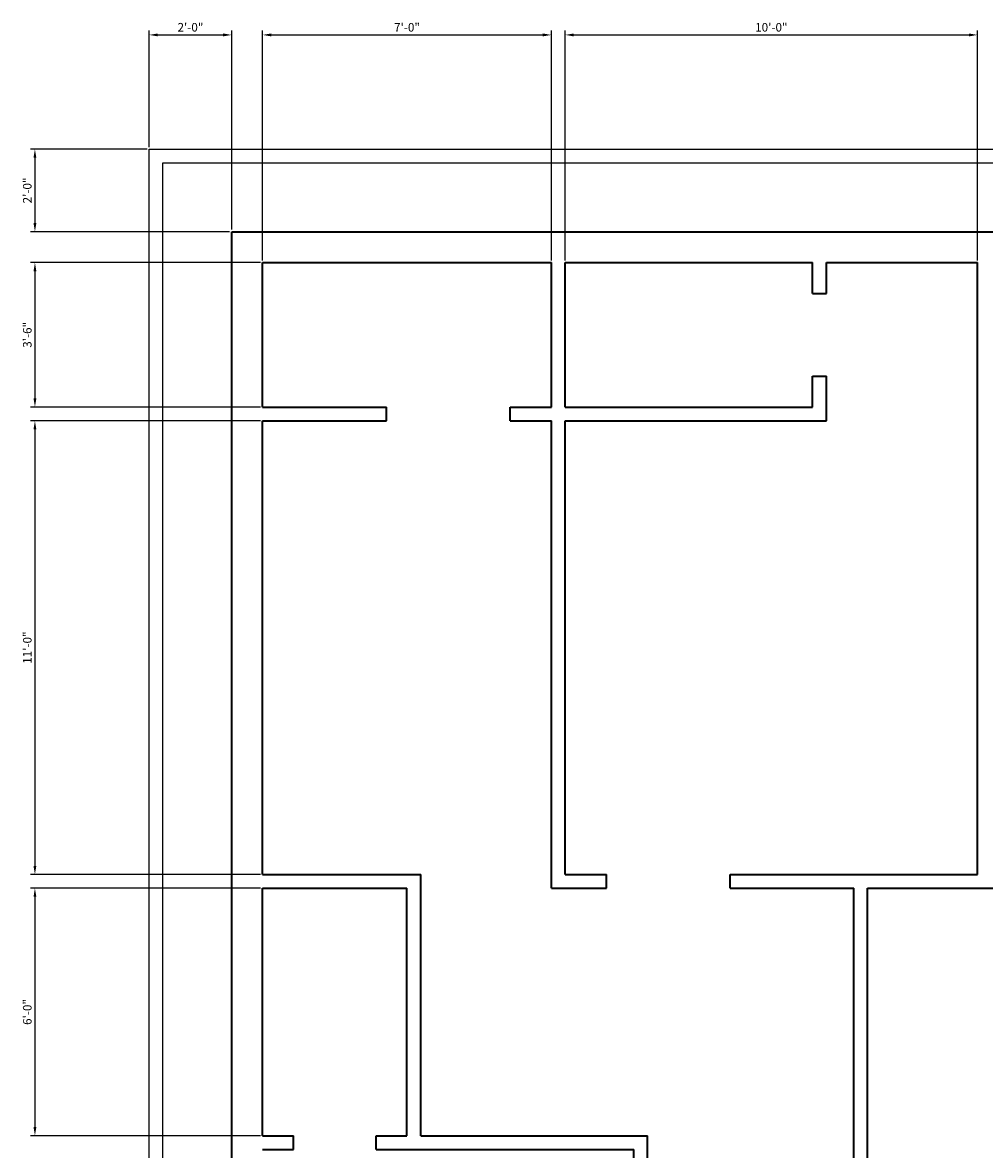
# Model space of a CAD drawing. Units: inches. Extents: x 2169 to 10664, y 1669 to 6352.
# Tile 11 of 17: x 4397 to 4677, y 2329 to 2657. Entities that reach past the tile are written whole.
import ezdxf

# ---------------------------------------------------------------- set-up
doc = ezdxf.new("R2010")
doc.units = ezdxf.units.IN
for name, color, linetype, lineweight in [('A-ANNO-DIMS', 3, 'Continuous', 18), ('A-WALL', 7, 'Continuous', 35), ('C-PROP', 251, 'Continuous', 25)]:
    doc.layers.add(name, color=color, linetype=linetype, lineweight=lineweight)
doc.styles.get("Standard").update_dxf_attribs({"font": 'arial.ttf'})
doc.dimstyles.new('ISO-25', dxfattribs={"dimtxt": 2.5, "dimasz": 2.5, "dimexe": 1.25, "dimexo": 0.625, "dimtad": 1, "dimdec": 0, "dimlunit": 3, "dimtxsty": 'Standard', "dimcen": 2.5, "dimadec": 0, "dimazin": 0, "dimtfac": 1, "dimtdec": 0, "dimtmove": 0, "dimatfit": 3, "dimfxl": 1, "dimarcsym": 0})

# ---------------------------------------------------------------- blocks, each defined once
blk = doc.blocks.new('*D104')
at = {"layer": 'A-ANNO-DIMS', "color": 0, "lineweight": -2, "transparency": 16777216}
for p, q in [((4433.57, 2620.81), (4433.57, 2654.69)), ((4436.07, 2653.44), (4455.07, 2653.44)), ((4457.57, 2596.81), (4457.57, 2654.69))]:
    blk.add_line(p, q, dxfattribs=at)
at = {"layer": 'A-ANNO-DIMS', "color": 0, "transparency": 16777216}
for points in [[(4436.07, 2653.86), (4436.07, 2653.02), (4433.57, 2653.44)], [(4455.07, 2653.86), (4455.07, 2653.02), (4457.57, 2653.44)]]:
    blk.add_solid(points, dxfattribs=at)
at = {"layer": 'Defpoints', "color": 0, "transparency": 16777216}
for p in [(4457.57, 2653.44), (4433.57, 2620.19), (4457.57, 2596.19)]:
    blk.add_point(p, dxfattribs=at)
at = {"layer": 'A-ANNO-DIMS', "color": 0, "transparency": 16777216, "insert": (4445.57, 2655.34), "char_height": 2.5, "attachment_point": 5}
blk.add_mtext('2\'-0"', dxfattribs=at)
blk = doc.blocks.new('*D105')
at = {"layer": 'A-ANNO-DIMS', "color": 0, "lineweight": -2, "transparency": 16777216}
for p, q in [((4466.57, 2587.81), (4466.57, 2654.69)), ((4469.07, 2653.44), (4548.07, 2653.44)), ((4550.57, 2587.81), (4550.57, 2654.69))]:
    blk.add_line(p, q, dxfattribs=at)
at = {"layer": 'A-ANNO-DIMS', "color": 0, "transparency": 16777216}
for points in [[(4469.07, 2653.86), (4469.07, 2653.02), (4466.57, 2653.44)], [(4548.07, 2653.86), (4548.07, 2653.02), (4550.57, 2653.44)]]:
    blk.add_solid(points, dxfattribs=at)
at = {"layer": 'Defpoints', "color": 0, "transparency": 16777216}
for p in [(4550.57, 2653.44), (4466.57, 2587.19), (4550.57, 2587.19)]:
    blk.add_point(p, dxfattribs=at)
at = {"layer": 'A-ANNO-DIMS', "color": 0, "transparency": 16777216, "insert": (4508.57, 2655.34), "char_height": 2.5, "attachment_point": 5}
blk.add_mtext('7\'-0"', dxfattribs=at)
blk = doc.blocks.new('*D106')
at = {"layer": 'A-ANNO-DIMS', "color": 0, "lineweight": -2, "transparency": 16777216}
for p, q in [((4554.57, 2587.81), (4554.57, 2654.69)), ((4557.07, 2653.44), (4672.07, 2653.44)), ((4674.57, 2587.81), (4674.57, 2654.69))]:
    blk.add_line(p, q, dxfattribs=at)
at = {"layer": 'A-ANNO-DIMS', "color": 0, "transparency": 16777216}
for points in [[(4557.07, 2653.86), (4557.07, 2653.02), (4554.57, 2653.44)], [(4672.07, 2653.86), (4672.07, 2653.02), (4674.57, 2653.44)]]:
    blk.add_solid(points, dxfattribs=at)
at = {"layer": 'Defpoints', "color": 0, "transparency": 16777216}
for p in [(4674.57, 2653.44), (4554.57, 2587.19), (4674.57, 2587.19)]:
    blk.add_point(p, dxfattribs=at)
at = {"layer": 'A-ANNO-DIMS', "color": 0, "transparency": 16777216, "insert": (4614.57, 2655.34), "char_height": 2.5, "attachment_point": 5}
blk.add_mtext('10\'-0"', dxfattribs=at)
blk = doc.blocks.new('*D110')
at = {"layer": 'A-ANNO-DIMS', "color": 0, "lineweight": -2, "transparency": 16777216}
for p, q in [((4432.95, 2620.19), (4399.07, 2620.19)), ((4400.32, 2617.69), (4400.32, 2598.69)), ((4456.95, 2596.19), (4399.07, 2596.19))]:
    blk.add_line(p, q, dxfattribs=at)
at = {"layer": 'A-ANNO-DIMS', "color": 0, "transparency": 16777216}
for points in [[(4399.91, 2617.69), (4400.74, 2617.69), (4400.32, 2620.19)], [(4399.91, 2598.69), (4400.74, 2598.69), (4400.32, 2596.19)]]:
    blk.add_solid(points, dxfattribs=at)
at = {"layer": 'Defpoints', "color": 0, "transparency": 16777216}
for p in [(4433.57, 2620.19), (4400.32, 2596.19), (4457.57, 2596.19)]:
    blk.add_point(p, dxfattribs=at)
at = {"layer": 'A-ANNO-DIMS', "color": 0, "transparency": 16777216, "insert": (4398.42, 2608.19), "char_height": 2.5, "attachment_point": 5, "rotation": 90}
blk.add_mtext('2\'-0"', dxfattribs=at)
blk = doc.blocks.new('*D111')
at = {"layer": 'A-ANNO-DIMS', "color": 0, "lineweight": -2, "transparency": 16777216}
for p, q in [((4465.95, 2587.19), (4399.07, 2587.19)), ((4400.32, 2584.69), (4400.32, 2547.69)), ((4465.95, 2545.19), (4399.07, 2545.19))]:
    blk.add_line(p, q, dxfattribs=at)
at = {"layer": 'A-ANNO-DIMS', "color": 0, "transparency": 16777216}
for points in [[(4399.91, 2584.69), (4400.74, 2584.69), (4400.32, 2587.19)], [(4399.91, 2547.69), (4400.74, 2547.69), (4400.32, 2545.19)]]:
    blk.add_solid(points, dxfattribs=at)
at = {"layer": 'Defpoints', "color": 0, "transparency": 16777216}
for p in [(4466.57, 2587.19), (4400.32, 2545.19), (4466.57, 2545.19)]:
    blk.add_point(p, dxfattribs=at)
at = {"layer": 'A-ANNO-DIMS', "color": 0, "transparency": 16777216, "insert": (4398.42, 2566.19), "char_height": 2.5, "attachment_point": 5, "rotation": 90}
blk.add_mtext('3\'-6"', dxfattribs=at)
blk = doc.blocks.new('*D112')
at = {"layer": 'A-ANNO-DIMS', "color": 0, "lineweight": -2, "transparency": 16777216}
for p, q in [((4465.95, 2541.19), (4399.07, 2541.19)), ((4400.32, 2538.69), (4400.32, 2411.69)), ((4465.95, 2409.19), (4399.07, 2409.19))]:
    blk.add_line(p, q, dxfattribs=at)
at = {"layer": 'A-ANNO-DIMS', "color": 0, "transparency": 16777216}
for points in [[(4399.91, 2538.69), (4400.74, 2538.69), (4400.32, 2541.19)], [(4399.91, 2411.69), (4400.74, 2411.69), (4400.32, 2409.19)]]:
    blk.add_solid(points, dxfattribs=at)
at = {"layer": 'Defpoints', "color": 0, "transparency": 16777216}
for p in [(4466.57, 2541.19), (4400.32, 2409.19), (4466.57, 2409.19)]:
    blk.add_point(p, dxfattribs=at)
at = {"layer": 'A-ANNO-DIMS', "color": 0, "transparency": 16777216, "insert": (4398.42, 2475.19), "char_height": 2.5, "attachment_point": 5, "rotation": 90}
blk.add_mtext('11\'-0"', dxfattribs=at)
blk = doc.blocks.new('*D113')
at = {"layer": 'A-ANNO-DIMS', "color": 0, "lineweight": -2, "transparency": 16777216}
for p, q in [((4465.95, 2405.19), (4399.07, 2405.19)), ((4400.32, 2402.69), (4400.32, 2335.69)), ((4465.95, 2333.19), (4399.07, 2333.19))]:
    blk.add_line(p, q, dxfattribs=at)
at = {"layer": 'A-ANNO-DIMS', "color": 0, "transparency": 16777216}
for points in [[(4399.91, 2402.69), (4400.74, 2402.69), (4400.32, 2405.19)], [(4399.91, 2335.69), (4400.74, 2335.69), (4400.32, 2333.19)]]:
    blk.add_solid(points, dxfattribs=at)
at = {"layer": 'Defpoints', "color": 0, "transparency": 16777216}
for p in [(4466.57, 2405.19), (4400.32, 2333.19), (4466.57, 2333.19)]:
    blk.add_point(p, dxfattribs=at)
at = {"layer": 'A-ANNO-DIMS', "color": 0, "transparency": 16777216, "insert": (4398.42, 2369.19), "char_height": 2.5, "attachment_point": 5, "rotation": 90}
blk.add_mtext('6\'-0"', dxfattribs=at)

msp = doc.modelspace()

# ---------------------------------------------------------------- linework, layer by layer
at = {"layer": 'A-WALL'}
for p, q in [((4457.57, 2059.19), (4457.57, 2596.19)), ((4457.57, 2596.19), (4889.57, 2596.19)), ((4466.57, 2587.19), (4550.57, 2587.19)), ((4466.57, 2545.19), (4466.57, 2587.19)), ((4550.57, 2545.19), (4550.57, 2587.19)), ((4554.57, 2587.19), (4626.57, 2587.19)), ((4554.57, 2545.19), (4554.57, 2587.19)), ((4626.57, 2578.19), (4626.57, 2587.19)), ((4630.57, 2578.19), (4630.57, 2587.19)), ((4630.57, 2587.19), (4674.57, 2587.19)), ((4674.57, 2409.19), (4674.57, 2587.19)), ((4626.57, 2578.19), (4630.57, 2578.19)), ((4626.57, 2545.19), (4626.57, 2554.19)), ((4626.57, 2554.19), (4630.57, 2554.19)), ((4630.57, 2541.19), (4630.57, 2554.19)), ((4466.57, 2545.19), (4502.57, 2545.19)), ((4502.57, 2541.19), (4502.57, 2545.19)), ((4538.57, 2541.19), (4538.57, 2545.19)), ((4538.57, 2545.19), (4550.57, 2545.19)), ((4554.57, 2545.19), (4626.57, 2545.19)), ((4466.57, 2541.19), (4502.57, 2541.19)), ((4466.57, 2409.19), (4466.57, 2541.19)), ((4538.57, 2541.19), (4550.57, 2541.19)), ((4550.57, 2405.19), (4550.57, 2541.19)), ((4554.57, 2409.19), (4554.57, 2541.19)), ((4554.57, 2541.19), (4630.57, 2541.19)), ((4466.57, 2409.19), (4512.57, 2409.19)), ((4512.57, 2333.19), (4512.57, 2409.19)), ((4554.57, 2409.19), (4566.57, 2409.19)), ((4566.57, 2405.19), (4566.57, 2409.19)), ((4602.57, 2405.19), (4602.57, 2409.19)), ((4602.57, 2409.19), (4674.57, 2409.19)), ((4466.57, 2405.19), (4508.57, 2405.19)), ((4466.57, 2333.19), (4466.57, 2405.19)), ((4508.57, 2333.19), (4508.57, 2405.19)), ((4550.57, 2405.19), (4566.57, 2405.19)), ((4602.57, 2405.19), (4638.57, 2405.19)), ((4638.57, 2185.19), (4638.57, 2405.19)), ((4642.57, 2189.19), (4642.57, 2405.19)), ((4642.57, 2405.19), (4726.57, 2405.19)), ((4466.57, 2333.19), (4475.57, 2333.19)), ((4475.57, 2329.19), (4475.57, 2333.19)), ((4499.57, 2329.19), (4499.57, 2333.19)), ((4499.57, 2333.19), (4508.57, 2333.19)), ((4512.57, 2333.19), (4578.57, 2333.19)), ((4578.57, 2185.19), (4578.57, 2333.19)), ((4466.57, 2329.19), (4475.57, 2329.19)), ((4499.57, 2329.19), (4574.57, 2329.19)), ((4574.57, 2189.19), (4574.57, 2329.19))]:
    msp.add_line(p, q, dxfattribs=at)
at = {"layer": 'C-PROP'}
for p, q in [((4433.57, 2620.19), (4913.57, 2620.19)), ((4433.57, 2002.19), (4433.57, 2620.19)), ((4437.57, 2011.19), (4437.57, 2616.19)), ((4437.57, 2616.19), (4909.57, 2616.19))]:
    msp.add_line(p, q, dxfattribs=at)

# ---------------------------------------------------------------- dimensions: what is measured, and where the dimension line sits
at = {"layer": 'A-ANNO-DIMS'}
for base, p1, p2, picture, middle in [((4457.57, 2653.44), (4433.57, 2620.19), (4457.57, 2596.19), '*D104', (4445.57, 2655.34)), ((4550.57, 2653.44), (4466.57, 2587.19), (4550.57, 2587.19), '*D105', (4508.57, 2655.34)), ((4674.57, 2653.44), (4554.57, 2587.19), (4674.57, 2587.19), '*D106', (4614.57, 2655.34))]:
    dim = msp.add_linear_dim(base=base, p1=p1, p2=p2, dimstyle='ISO-25', override={"dimdec": 1, "dimlfac": 1, "dimrnd": 0, "dimzin": 1, "dimdsep": 46, "dimlunit": 4, "dimfrac": 2}, dxfattribs=at)
    dim.commit()
    dim.dimension.update_dxf_attribs({"geometry": picture, "text_midpoint": middle})
for base, p1, p2, picture, middle in [((4400.32, 2596.19), (4433.57, 2620.19), (4457.57, 2596.19), '*D110', (4398.42, 2608.19)), ((4400.32, 2545.19), (4466.57, 2587.19), (4466.57, 2545.19), '*D111', (4398.42, 2566.19)), ((4400.32, 2409.19), (4466.57, 2541.19), (4466.57, 2409.19), '*D112', (4398.42, 2475.19)), ((4400.32, 2333.19), (4466.57, 2405.19), (4466.57, 2333.19), '*D113', (4398.42, 2369.19))]:
    dim = msp.add_linear_dim(base=base, p1=p1, p2=p2, angle=90, dimstyle='ISO-25', override={"dimdec": 1, "dimlfac": 1, "dimrnd": 0, "dimzin": 1, "dimdsep": 46, "dimlunit": 4, "dimfrac": 2}, dxfattribs=at)
    dim.commit()
    dim.dimension.update_dxf_attribs({"geometry": picture, "text_midpoint": middle})

doc.saveas('drawing.dxf')
